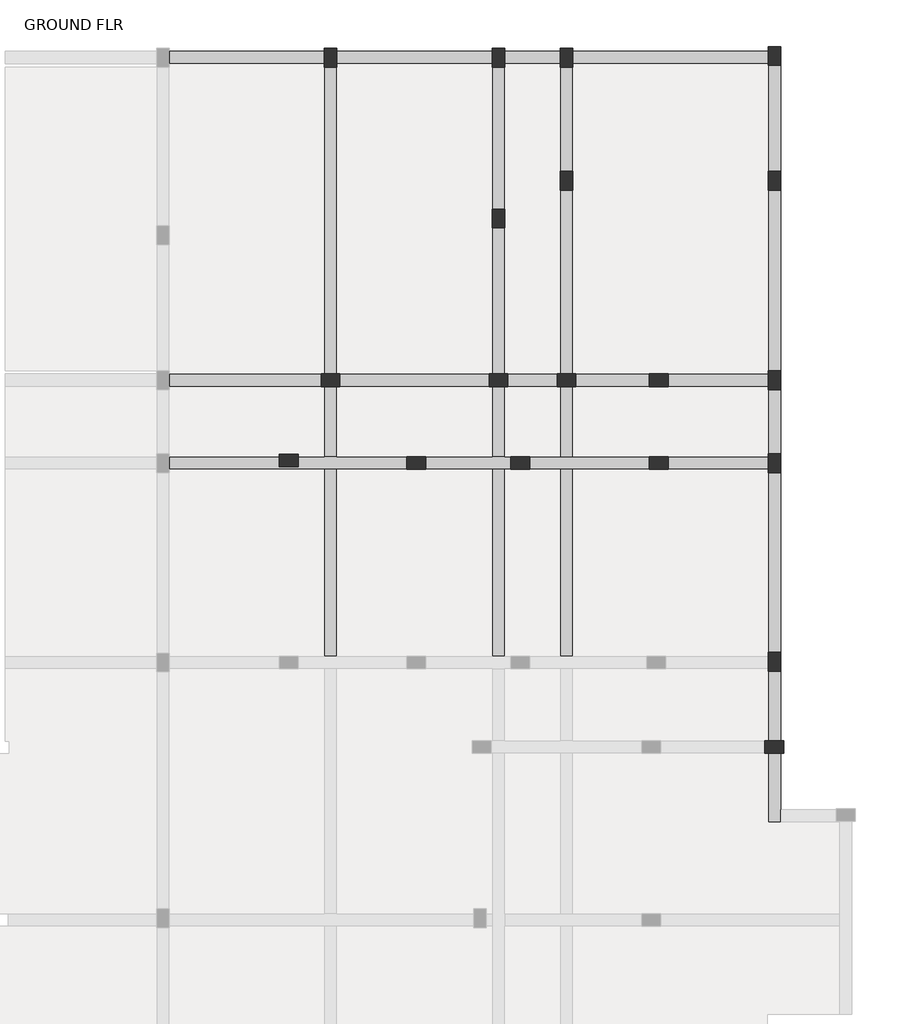
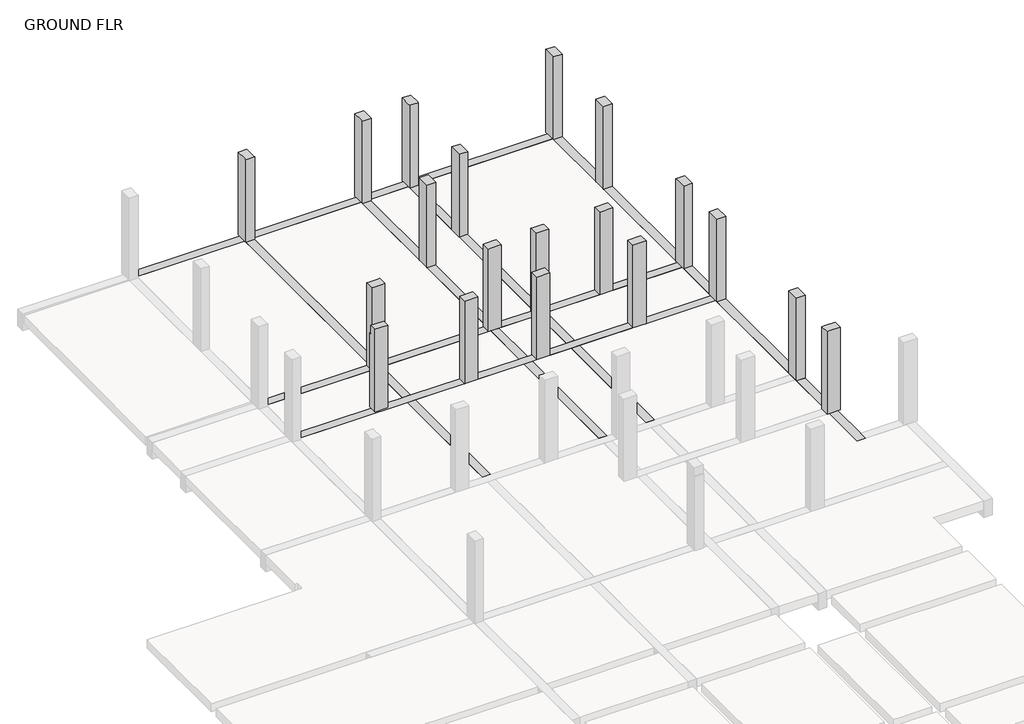
# One storey, part 5 of 5: 30 beams, 19 columns.
"""IFC4 building model written with IfcOpenShell, lengths in millimetres."""

from ifc_helpers import new_model, si_unit, frame, origin, origin_with_axes, place, context, project, spatial, polyline, outline, extrude, faceted_brep, element, save

model = new_model("IFC4")

# Units and contexts
model_context = context("Model", 3, world=origin())
ifc_project = project(units=[si_unit("LENGTHUNIT", "METRE", prefix="MILLI")], contexts=[model_context])

# Site, building, storey
site = spatial("IfcSite", under=ifc_project)
building = spatial("IfcBuilding", under=site)
storey = spatial("IfcBuildingStorey", under=building, Name="GROUND FLR", Elevation=0.0)

# Beams
placement = place(None, origin())
element("IfcBeam", 1, ObjectType="M_Concrete-Rectangular Beam : 300 x 600mm", at=placement, inside=storey, context=model_context, shape_type="Brep", body=[
    faceted_brep([(2024.7296816, 21537.8349362, 0.0), (2024.7296816, 21837.8349362, 0.0), (-1671.7865686, 21837.8349362, 0.0), (-1671.7865686, 21537.8349362, 0.0), (2024.7296816, 21537.8349362, -600.0), (2024.7296816, 21537.8349362, -300.0), (-1671.7865686, 21537.8349362, -300.0), (-1671.7865686, 21537.8349362, -600.0), (2024.7296816, 21837.8349362, -600.0), (-1671.7865686, 21837.8349362, -600.0)], [[[0, 1, 2, 3]], [[4, 5, 0, 3, 6, 7]], [[8, 4, 7, 9]], [[1, 8, 9, 2]], [[2, 9, 7, 6, 3]], [[1, 0, 5, 4, 8]]]),
])
element("IfcBeam", 2, ObjectType="M_Concrete-Rectangular Beam : 300 x 600mm", at=placement, inside=storey, context=model_context, shape_type="Brep", body=[
    faceted_brep([(6032.5248054, 21537.8349362, 0.0), (6032.5248054, 21837.8349362, 0.0), (2324.7296816, 21837.8349362, 0.0), (2324.7296816, 21537.8349362, 0.0), (6032.5248054, 21537.8349362, -600.0), (6032.5248054, 21537.8349362, -300.0), (2324.7296816, 21537.8349362, -300.0), (2324.7296816, 21537.8349362, -600.0), (6032.5248054, 21837.8349362, -600.0), (2324.7296816, 21837.8349362, -600.0)], [[[0, 1, 2, 3]], [[4, 5, 0, 3, 6, 7]], [[8, 4, 7, 9]], [[1, 8, 9, 2]], [[2, 9, 7, 6, 3]], [[1, 0, 5, 4, 8]]]),
])
element("IfcBeam", 3, ObjectType="M_Concrete-Rectangular Beam : 300 x 600mm", at=placement, inside=storey, context=model_context, shape_type="Brep", body=[
    faceted_brep([(7656.8679014, 21537.8349362, 0.0), (7656.8679014, 21837.8349362, 0.0), (6332.5248054, 21837.8349362, 0.0), (6332.5248054, 21537.8349362, 0.0), (7656.8679014, 21537.8349362, -600.0), (7656.8679014, 21537.8349362, -300.0), (6332.5248054, 21537.8349362, -300.0), (6332.5248054, 21537.8349362, -600.0), (7656.8679014, 21837.8349362, -600.0), (6332.5248054, 21837.8349362, -600.0)], [[[0, 1, 2, 3]], [[4, 5, 0, 3, 6, 7]], [[8, 4, 7, 9]], [[1, 8, 9, 2]], [[2, 9, 7, 6, 3]], [[1, 0, 5, 4, 8]]]),
])
element("IfcBeam", 4, ObjectType="M_Concrete-Rectangular Beam : 300 x 600mm", at=placement, inside=storey, context=model_context, shape_type="Brep", body=[
    faceted_brep([(7956.8679014, 21837.8349362, 0.0), (7956.8679014, 21537.8349362, 0.0), (12619.1163908, 21537.8349362, 0.0), (12619.1163908, 21837.8349362, 0.0), (7956.8679014, 21537.8349362, -300.0), (7956.8679014, 21537.8349362, -600.0), (12619.1163908, 21537.8349362, -600.0), (12619.1163908, 21537.8349362, -300.0), (7956.8679014, 21837.8349362, -600.0), (12619.1163908, 21837.8349362, -600.0)], [[[0, 1, 2, 3]], [[1, 4, 5, 6, 7, 2]], [[5, 8, 9, 6]], [[8, 0, 3, 9]], [[0, 8, 5, 4, 1]], [[3, 2, 7, 6, 9]]]),
])
element("IfcBeam", 5, ObjectType="M_Concrete-Rectangular Beam : 300 x 600mm", at=placement, inside=storey, context=model_context, shape_type="Brep", body=[
    faceted_brep([(12916.8679014, 5087.6057249, 0.0), (12616.8679014, 5087.6057249, 0.0), (12616.8679014, 3435.7536525, 0.0), (12916.8679014, 3435.7536525, 0.0), (12916.8679014, 3735.7536525, 0.0), (12616.8679014, 5087.6057249, -300.0), (12616.8679014, 5087.6057249, -600.0), (12616.8679014, 3435.7536525, -600.0), (12616.8679014, 3435.7536525, -300.0), (12916.8679014, 5087.6057249, -600.0), (12916.8679014, 3735.7536525, -600.0), (12916.8679014, 3435.7536525, -600.0), (12916.8679014, 3435.7536525, -300.0)], [[[0, 1, 2, 3, 4]], [[2, 1, 5, 6, 7, 8]], [[6, 9, 10, 11, 7]], [[9, 0, 4, 3, 12, 11, 10]], [[0, 9, 6, 5, 1]], [[3, 2, 8, 7, 11, 12]]]),
])
element("IfcBeam", 6, ObjectType="M_Concrete-Rectangular Beam : 300 x 600mm", at=placement, inside=storey, context=model_context, shape_type="Brep", body=[
    faceted_brep([(12616.8679014, 5387.6057249, 0.0), (12916.8679014, 5387.6057249, 0.0), (12916.8679014, 7044.7076276, 0.0), (12619.1163908, 7044.7076276, 0.0), (12619.1163908, 7399.7076276, 0.0), (12616.8679014, 7399.7076276, 0.0), (12616.8679014, 7099.7076276, 0.0), (12616.8679014, 7399.7076276, -600.0), (12616.8679014, 7099.7076276, -600.0), (12616.8679014, 5387.6057249, -600.0), (12616.8679014, 5387.6057249, -300.0), (12616.8679014, 7399.7076276, -300.0), (12916.8679014, 5387.6057249, -600.0), (12619.1163908, 7399.7076276, -600.0), (12619.1163908, 7044.7076276, -600.0), (12916.8679014, 7044.7076276, -600.0)], [[[0, 1, 2, 3, 4, 5, 6]], [[7, 8, 9, 10, 0, 6, 5, 11]], [[12, 9, 8, 7, 13, 14, 15]], [[1, 12, 15, 2]], [[1, 0, 10, 9, 12]], [[14, 3, 2, 15]], [[3, 14, 13, 4]], [[5, 4, 13, 7, 11]]]),
])
element("IfcBeam", 7, ObjectType="M_Concrete-Rectangular Beam : 300 x 600mm", at=placement, inside=storey, context=model_context, shape_type="SweptSolid", body=[
    extrude(outline(polyline([(12619.1163908, 11782.4075451), (12919.1163908, 11782.4075451), (12919.1163908, 7494.7076276), (12619.1163908, 7494.7076276), (12619.1163908, 11782.4075451)])), frame((0.0, 0.0, -600.0), z_axis=(0.0, 0.0, 1.0), x_axis=(1.0, 0.0, 0.0)), (0.0, 0.0, 1.0), 600.0),
])
element("IfcBeam", 8, ObjectType="M_Concrete-Rectangular Beam : 300 x 600mm", at=placement, inside=storey, context=model_context, shape_type="Brep", body=[
    faceted_brep([(12619.1163908, 13762.5179708, 0.0), (12619.1163908, 12232.4075451, 0.0), (12919.1163908, 12232.4075451, 0.0), (12919.1163908, 13762.5179708, 0.0), (12919.1163908, 12232.4075451, -600.0), (12919.1163908, 13762.5179708, -600.0), (12619.1163908, 12232.4075451, -600.0), (12619.1163908, 13762.5179708, -600.0), (12619.1163908, 13762.5179708, -300.0), (12619.1163908, 12232.4075451, -300.0)], [[[0, 1, 2, 3]], [[3, 2, 4, 5]], [[5, 4, 6, 7]], [[1, 0, 8, 7, 6, 9]], [[0, 3, 5, 7, 8]], [[6, 4, 2, 1, 9]]]),
])
element("IfcBeam", 9, ObjectType="M_Concrete-Rectangular Beam : 300 x 600mm", at=placement, inside=storey, context=model_context, shape_type="Brep", body=[
    faceted_brep([(12619.1163908, 18524.7148651, 0.0), (12619.1163908, 14212.5179708, 0.0), (12919.1163908, 14212.5179708, 0.0), (12919.1163908, 18524.7148651, 0.0), (12919.1163908, 14212.5179708, -600.0), (12919.1163908, 18524.7148651, -600.0), (12619.1163908, 14212.5179708, -600.0), (12619.1163908, 18524.7148651, -600.0), (12619.1163908, 18524.7148651, -300.0), (12619.1163908, 14212.5179708, -300.0)], [[[0, 1, 2, 3]], [[3, 2, 4, 5]], [[5, 4, 6, 7]], [[1, 0, 8, 7, 6, 9]], [[0, 3, 5, 7, 8]], [[6, 4, 2, 1, 9]]]),
])
element("IfcBeam", 10, ObjectType="M_Concrete-Rectangular Beam : 300 x 600mm", at=placement, inside=storey, context=model_context, shape_type="Brep", body=[
    faceted_brep([(12619.1163908, 21502.8349362, 0.0), (12619.1163908, 18974.7148651, 0.0), (12919.1163908, 18974.7148651, 0.0), (12919.1163908, 21502.8349362, 0.0), (12919.1163908, 18974.7148651, -600.0), (12919.1163908, 21502.8349362, -600.0), (12619.1163908, 18974.7148651, -600.0), (12619.1163908, 21502.8349362, -600.0), (12619.1163908, 21502.8349362, -300.0), (12619.1163908, 18974.7148651, -300.0)], [[[0, 1, 2, 3]], [[3, 2, 4, 5]], [[5, 4, 6, 7]], [[1, 0, 8, 7, 6, 9]], [[6, 4, 2, 1, 9]], [[0, 3, 5, 7, 8]]]),
])
element("IfcBeam", 11, ObjectType="M_Concrete-Rectangular Beam : 300 x 600mm", at=placement, inside=storey, context=model_context, shape_type="Brep", body=[
    faceted_brep([(2324.7296816, 21462.8349362, 0.0), (2024.7296816, 21462.8349362, 0.0), (2024.7296816, 14137.5179708, 0.0), (2324.7296816, 14137.5179708, 0.0), (2024.7296816, 21462.8349362, -300.0), (2024.7296816, 21462.8349362, -600.0), (2024.7296816, 14137.5179708, -600.0), (2024.7296816, 14137.5179708, -300.0), (2324.7296816, 21462.8349362, -600.0), (2324.7296816, 14137.5179708, -600.0), (2324.7296816, 14137.5179708, -300.0), (2324.7296816, 21462.8349362, -300.0)], [[[0, 1, 2, 3]], [[2, 1, 4, 5, 6, 7]], [[5, 8, 9, 6]], [[0, 3, 10, 9, 8, 11]], [[1, 0, 11, 8, 5, 4]], [[3, 2, 7, 6, 9, 10]]]),
])
element("IfcBeam", 12, ObjectType="M_Concrete-Rectangular Beam : 300 x 600mm", at=placement, inside=storey, context=model_context, shape_type="Brep", body=[
    faceted_brep([(2324.7296816, 13837.5179708, 0.0), (2024.7296816, 13837.5179708, 0.0), (2024.7296816, 12157.4075451, 0.0), (2324.7296816, 12157.4075451, 0.0), (2024.7296816, 13837.5179708, -300.0), (2024.7296816, 13837.5179708, -600.0), (2024.7296816, 12157.4075451, -600.0), (2024.7296816, 12157.4075451, -300.0), (2324.7296816, 13837.5179708, -600.0), (2324.7296816, 12157.4075451, -600.0), (2324.7296816, 12157.4075451, -300.0), (2324.7296816, 13837.5179708, -300.0)], [[[0, 1, 2, 3]], [[2, 1, 4, 5, 6, 7]], [[5, 8, 9, 6]], [[0, 3, 10, 9, 8, 11]], [[1, 0, 11, 8, 5, 4]], [[3, 2, 7, 6, 9, 10]]]),
])
element("IfcBeam", 13, ObjectType="M_Concrete-Rectangular Beam : 300 x 600mm", at=placement, inside=storey, context=model_context, shape_type="Brep", body=[
    faceted_brep([(6332.5248054, 21462.8349362, 0.0), (6032.5248054, 21462.8349362, 0.0), (6032.5248054, 18074.7148651, 0.0), (6332.5248054, 18074.7148651, 0.0), (6032.5248054, 21462.8349362, -300.0), (6032.5248054, 21462.8349362, -600.0), (6032.5248054, 18074.7148651, -600.0), (6032.5248054, 18074.7148651, -300.0), (6332.5248054, 21462.8349362, -600.0), (6332.5248054, 18074.7148651, -600.0), (6332.5248054, 18074.7148651, -300.0), (6332.5248054, 21462.8349362, -300.0)], [[[0, 1, 2, 3]], [[2, 1, 4, 5, 6, 7]], [[5, 8, 9, 6]], [[0, 3, 10, 9, 8, 11]], [[1, 0, 11, 8, 5, 4]], [[3, 2, 7, 6, 9, 10]]]),
])
element("IfcBeam", 14, ObjectType="M_Concrete-Rectangular Beam : 300 x 600mm", at=placement, inside=storey, context=model_context, shape_type="Brep", body=[
    faceted_brep([(6332.5248054, 17624.7148651, 0.0), (6032.5248054, 17624.7148651, 0.0), (6032.5248054, 14137.5179708, 0.0), (6332.5248054, 14137.5179708, 0.0), (6032.5248054, 17624.7148651, -300.0), (6032.5248054, 17624.7148651, -600.0), (6032.5248054, 14137.5179708, -600.0), (6032.5248054, 14137.5179708, -300.0), (6332.5248054, 17624.7148651, -600.0), (6332.5248054, 14137.5179708, -600.0), (6332.5248054, 14137.5179708, -300.0), (6332.5248054, 17624.7148651, -300.0)], [[[0, 1, 2, 3]], [[2, 1, 4, 5, 6, 7]], [[5, 8, 9, 6]], [[0, 3, 10, 9, 8, 11]], [[1, 0, 11, 8, 5, 4]], [[3, 2, 7, 6, 9, 10]]]),
])
element("IfcBeam", 15, ObjectType="M_Concrete-Rectangular Beam : 300 x 600mm", at=placement, inside=storey, context=model_context, shape_type="Brep", body=[
    faceted_brep([(6332.5248054, 13837.5179708, 0.0), (6032.5248054, 13837.5179708, 0.0), (6032.5248054, 12157.4075451, 0.0), (6332.5248054, 12157.4075451, 0.0), (6032.5248054, 13837.5179708, -300.0), (6032.5248054, 13837.5179708, -600.0), (6032.5248054, 12157.4075451, -600.0), (6032.5248054, 12157.4075451, -300.0), (6332.5248054, 13837.5179708, -600.0), (6332.5248054, 12157.4075451, -600.0), (6332.5248054, 12157.4075451, -300.0), (6332.5248054, 13837.5179708, -300.0)], [[[0, 1, 2, 3]], [[2, 1, 4, 5, 6, 7]], [[5, 8, 9, 6]], [[0, 3, 10, 9, 8, 11]], [[1, 0, 11, 8, 5, 4]], [[3, 2, 7, 6, 9, 10]]]),
])
element("IfcBeam", 16, ObjectType="M_Concrete-Rectangular Beam : 300 x 600mm", at=placement, inside=storey, context=model_context, shape_type="Brep", body=[
    faceted_brep([(7956.8679014, 21462.8349362, 0.0), (7656.8679014, 21462.8349362, 0.0), (7656.8679014, 18974.7148651, 0.0), (7956.8679014, 18974.7148651, 0.0), (7656.8679014, 21462.8349362, -300.0), (7656.8679014, 21462.8349362, -600.0), (7656.8679014, 18974.7148651, -600.0), (7656.8679014, 18974.7148651, -300.0), (7956.8679014, 21462.8349362, -600.0), (7956.8679014, 18974.7148651, -600.0), (7956.8679014, 18974.7148651, -300.0), (7956.8679014, 21462.8349362, -300.0)], [[[0, 1, 2, 3]], [[2, 1, 4, 5, 6, 7]], [[5, 8, 9, 6]], [[0, 3, 10, 9, 8, 11]], [[1, 0, 11, 8, 5, 4]], [[3, 2, 7, 6, 9, 10]]]),
])
element("IfcBeam", 17, ObjectType="M_Concrete-Rectangular Beam : 300 x 600mm", at=placement, inside=storey, context=model_context, shape_type="Brep", body=[
    faceted_brep([(7956.8679014, 18524.7148651, 0.0), (7656.8679014, 18524.7148651, 0.0), (7656.8679014, 14137.5179708, 0.0), (7956.8679014, 14137.5179708, 0.0), (7656.8679014, 18524.7148651, -300.0), (7656.8679014, 18524.7148651, -600.0), (7656.8679014, 14137.5179708, -600.0), (7656.8679014, 14137.5179708, -300.0), (7956.8679014, 18524.7148651, -600.0), (7956.8679014, 14137.5179708, -600.0), (7956.8679014, 14137.5179708, -300.0), (7956.8679014, 18524.7148651, -300.0)], [[[0, 1, 2, 3]], [[2, 1, 4, 5, 6, 7]], [[5, 8, 9, 6]], [[0, 3, 10, 9, 8, 11]], [[1, 0, 11, 8, 5, 4]], [[3, 2, 7, 6, 9, 10]]]),
])
element("IfcBeam", 18, ObjectType="M_Concrete-Rectangular Beam : 300 x 600mm", at=placement, inside=storey, context=model_context, shape_type="Brep", body=[
    faceted_brep([(7956.8679014, 13837.5179708, 0.0), (7656.8679014, 13837.5179708, 0.0), (7656.8679014, 12157.4075451, 0.0), (7956.8679014, 12157.4075451, 0.0), (7656.8679014, 13837.5179708, -300.0), (7656.8679014, 13837.5179708, -600.0), (7656.8679014, 12157.4075451, -600.0), (7656.8679014, 12157.4075451, -300.0), (7956.8679014, 13837.5179708, -600.0), (7956.8679014, 12157.4075451, -600.0), (7956.8679014, 12157.4075451, -300.0), (7956.8679014, 13837.5179708, -300.0)], [[[0, 1, 2, 3]], [[2, 1, 4, 5, 6, 7]], [[5, 8, 9, 6]], [[0, 3, 10, 9, 8, 11]], [[1, 0, 11, 8, 5, 4]], [[3, 2, 7, 6, 9, 10]]]),
])
element("IfcBeam", 19, ObjectType="M_Concrete-Rectangular Beam : 300 x 600mm", at=placement, inside=storey, context=model_context, shape_type="Brep", body=[
    faceted_brep([(-1671.7865686, 14137.5179708, 0.0), (-1671.7865686, 13837.5179708, 0.0), (1949.7296816, 13837.5179708, 0.0), (1949.7296816, 14137.5179708, 0.0), (-1671.7865686, 13837.5179708, -300.0), (-1671.7865686, 13837.5179708, -600.0), (1949.7296816, 13837.5179708, -600.0), (1949.7296816, 13837.5179708, -300.0), (-1671.7865686, 14137.5179708, -600.0), (1949.7296816, 14137.5179708, -600.0), (1949.7296816, 14137.5179708, -300.0), (-1671.7865686, 14137.5179708, -300.0)], [[[0, 1, 2, 3]], [[2, 1, 4, 5, 6, 7]], [[5, 8, 9, 6]], [[0, 3, 10, 9, 8, 11]], [[1, 0, 11, 8, 5, 4]], [[3, 2, 7, 6, 9, 10]]]),
])
element("IfcBeam", 20, ObjectType="M_Concrete-Rectangular Beam : 300 x 600mm", at=placement, inside=storey, context=model_context, shape_type="Brep", body=[
    faceted_brep([(2399.7296816, 14137.5179708, 0.0), (2399.7296816, 13837.5179708, 0.0), (5957.5248054, 13837.5179708, 0.0), (5957.5248054, 14137.5179708, 0.0), (2399.7296816, 13837.5179708, -300.0), (2399.7296816, 13837.5179708, -600.0), (5957.5248054, 13837.5179708, -600.0), (5957.5248054, 13837.5179708, -300.0), (2399.7296816, 14137.5179708, -600.0), (5957.5248054, 14137.5179708, -600.0), (5957.5248054, 14137.5179708, -300.0), (2399.7296816, 14137.5179708, -300.0)], [[[0, 1, 2, 3]], [[2, 1, 4, 5, 6, 7]], [[5, 8, 9, 6]], [[0, 3, 10, 9, 8, 11]], [[1, 0, 11, 8, 5, 4]], [[3, 2, 7, 6, 9, 10]]]),
])
element("IfcBeam", 21, ObjectType="M_Concrete-Rectangular Beam : 300 x 600mm", at=placement, inside=storey, context=model_context, shape_type="Brep", body=[
    faceted_brep([(6407.5248054, 14137.5179708, 0.0), (6407.5248054, 13837.5179708, 0.0), (7581.8679014, 13837.5179708, 0.0), (7581.8679014, 14137.5179708, 0.0), (6407.5248054, 13837.5179708, -300.0), (6407.5248054, 13837.5179708, -600.0), (7581.8679014, 13837.5179708, -600.0), (7581.8679014, 13837.5179708, -300.0), (6407.5248054, 14137.5179708, -600.0), (7581.8679014, 14137.5179708, -600.0), (7581.8679014, 14137.5179708, -300.0), (6407.5248054, 14137.5179708, -300.0)], [[[0, 1, 2, 3]], [[2, 1, 4, 5, 6, 7]], [[5, 8, 9, 6]], [[0, 3, 10, 9, 8, 11]], [[1, 0, 11, 8, 5, 4]], [[3, 2, 7, 6, 9, 10]]]),
])
element("IfcBeam", 22, ObjectType="M_Concrete-Rectangular Beam : 300 x 600mm", at=placement, inside=storey, context=model_context, shape_type="Brep", body=[
    faceted_brep([(8031.8679014, 14137.5179708, 0.0), (8031.8679014, 13837.5179708, 0.0), (9781.8679014, 13837.5179708, 0.0), (9781.8679014, 14137.5179708, 0.0), (8031.8679014, 13837.5179708, -300.0), (8031.8679014, 13837.5179708, -600.0), (9781.8679014, 13837.5179708, -600.0), (9781.8679014, 13837.5179708, -300.0), (8031.8679014, 14137.5179708, -600.0), (9781.8679014, 14137.5179708, -600.0), (9781.8679014, 14137.5179708, -300.0), (8031.8679014, 14137.5179708, -300.0)], [[[0, 1, 2, 3]], [[2, 1, 4, 5, 6, 7]], [[5, 8, 9, 6]], [[0, 3, 10, 9, 8, 11]], [[1, 0, 11, 8, 5, 4]], [[3, 2, 7, 6, 9, 10]]]),
])
element("IfcBeam", 23, ObjectType="M_Concrete-Rectangular Beam : 300 x 600mm", at=placement, inside=storey, context=model_context, shape_type="Brep", body=[
    faceted_brep([(10231.8679014, 14137.5179708, 0.0), (10231.8679014, 13837.5179708, 0.0), (12619.1163908, 13837.5179708, 0.0), (12619.1163908, 14137.5179708, 0.0), (10231.8679014, 13837.5179708, -300.0), (10231.8679014, 13837.5179708, -600.0), (12619.1163908, 13837.5179708, -600.0), (12619.1163908, 13837.5179708, -300.0), (10231.8679014, 14137.5179708, -600.0), (12619.1163908, 14137.5179708, -600.0), (12619.1163908, 14137.5179708, -300.0), (10231.8679014, 14137.5179708, -300.0)], [[[0, 1, 2, 3]], [[2, 1, 4, 5, 6, 7]], [[5, 8, 9, 6]], [[0, 3, 10, 9, 8, 11]], [[1, 0, 11, 8, 5, 4]], [[3, 2, 7, 6, 9, 10]]]),
])
element("IfcBeam", 24, ObjectType="M_Concrete-Rectangular Beam : 300 x 600mm", at=placement, inside=storey, context=model_context, shape_type="Brep", body=[
    faceted_brep([(-1671.7865686, 12157.4075451, 0.0), (-1671.7865686, 11857.4075451, 0.0), (2024.7296816, 11857.4075451, 0.0), (2324.7296816, 11857.4075451, 0.0), (3997.5248054, 11857.4075451, 0.0), (3997.5248054, 12157.4075451, 0.0), (2324.7296816, 12157.4075451, 0.0), (2024.7296816, 12157.4075451, 0.0), (1399.7296816, 12157.4075451, 0.0), (1399.7296816, 11917.4075451, 0.0), (949.7296816, 11917.4075451, 0.0), (949.7296816, 12157.4075451, 0.0), (-1671.7865686, 11857.4075451, -600.0), (2024.7296816, 11857.4075451, -600.0), (2324.7296816, 11857.4075451, -600.0), (3997.5248054, 11857.4075451, -600.0), (3997.5248054, 11857.4075451, -300.0), (-1671.7865686, 11857.4075451, -300.0), (-1671.7865686, 12157.4075451, -600.0), (949.7296816, 12157.4075451, -600.0), (949.7296816, 11917.4075451, -600.0), (1399.7296816, 11917.4075451, -600.0), (1399.7296816, 12157.4075451, -600.0), (2024.7296816, 12157.4075451, -600.0), (2324.7296816, 12157.4075451, -600.0), (3997.5248054, 12157.4075451, -600.0), (949.7296816, 12157.4075451, -300.0), (-1671.7865686, 12157.4075451, -300.0), (3997.5248054, 12157.4075451, -300.0), (1399.7296816, 12157.4075451, -300.0)], [[[0, 1, 2, 3, 4, 5, 6, 7, 8, 9, 10, 11]], [[12, 13, 14, 15, 16, 4, 3, 2, 1, 17]], [[12, 18, 19, 20, 21, 22, 23, 24, 25, 15, 14, 13]], [[0, 11, 26, 19, 18, 27]], [[1, 0, 27, 18, 12, 17]], [[5, 4, 16, 15, 25, 28]], [[20, 10, 9, 21]], [[10, 20, 19, 26, 11]], [[21, 9, 8, 29, 22]], [[25, 24, 23, 22, 29, 8, 7, 6, 5, 28]]]),
])
element("IfcBeam", 25, ObjectType="M_Concrete-Rectangular Beam : 300 x 600mm", at=placement, inside=storey, context=model_context, shape_type="Brep", body=[
    faceted_brep([(4447.5248054, 12157.4075451, 0.0), (4447.5248054, 11857.4075451, 0.0), (6032.5248054, 11857.4075451, 0.0), (6332.5248054, 11857.4075451, 0.0), (6481.8679014, 11857.4075451, 0.0), (6481.8679014, 12157.4075451, 0.0), (6332.5248054, 12157.4075451, 0.0), (6032.5248054, 12157.4075451, 0.0), (4447.5248054, 11857.4075451, -600.0), (6032.5248054, 11857.4075451, -600.0), (6332.5248054, 11857.4075451, -600.0), (6481.8679014, 11857.4075451, -600.0), (6481.8679014, 11857.4075451, -300.0), (4447.5248054, 11857.4075451, -300.0), (4447.5248054, 12157.4075451, -600.0), (6032.5248054, 12157.4075451, -600.0), (6332.5248054, 12157.4075451, -600.0), (6481.8679014, 12157.4075451, -600.0), (4447.5248054, 12157.4075451, -300.0), (6481.8679014, 12157.4075451, -300.0)], [[[0, 1, 2, 3, 4, 5, 6, 7]], [[8, 9, 10, 11, 12, 4, 3, 2, 1, 13]], [[8, 14, 15, 16, 17, 11, 10, 9]], [[17, 16, 15, 14, 18, 0, 7, 6, 5, 19]], [[1, 0, 18, 14, 8, 13]], [[5, 4, 12, 11, 17, 19]]]),
])
element("IfcBeam", 26, ObjectType="M_Concrete-Rectangular Beam : 300 x 600mm", at=placement, inside=storey, context=model_context, shape_type="Brep", body=[
    faceted_brep([(6931.8679014, 12157.4075451, 0.0), (6931.8679014, 11857.4075451, 0.0), (7656.8679014, 11857.4075451, 0.0), (7956.8679014, 11857.4075451, 0.0), (9781.8679014, 11857.4075451, 0.0), (9781.8679014, 12157.4075451, 0.0), (7956.8679014, 12157.4075451, 0.0), (7656.8679014, 12157.4075451, 0.0), (6931.8679014, 11857.4075451, -600.0), (7656.8679014, 11857.4075451, -600.0), (7956.8679014, 11857.4075451, -600.0), (9781.8679014, 11857.4075451, -600.0), (9781.8679014, 11857.4075451, -300.0), (6931.8679014, 11857.4075451, -300.0), (6931.8679014, 12157.4075451, -600.0), (7656.8679014, 12157.4075451, -600.0), (7956.8679014, 12157.4075451, -600.0), (9781.8679014, 12157.4075451, -600.0), (6931.8679014, 12157.4075451, -300.0), (9781.8679014, 12157.4075451, -300.0)], [[[0, 1, 2, 3, 4, 5, 6, 7]], [[8, 9, 10, 11, 12, 4, 3, 2, 1, 13]], [[8, 14, 15, 16, 17, 11, 10, 9]], [[17, 16, 15, 14, 18, 0, 7, 6, 5, 19]], [[1, 0, 18, 14, 8, 13]], [[5, 4, 12, 11, 17, 19]]]),
])
element("IfcBeam", 27, ObjectType="M_Concrete-Rectangular Beam : 300 x 600mm", at=placement, inside=storey, context=model_context, shape_type="Brep", body=[
    faceted_brep([(10231.8679014, 12157.4075451, 0.0), (10231.8679014, 11857.4075451, 0.0), (12616.8679014, 11857.4075451, 0.0), (12619.1163908, 11857.4075451, 0.0), (12619.1163908, 12157.4075451, 0.0), (10231.8679014, 11857.4075451, -600.0), (12619.1163908, 11857.4075451, -600.0), (10231.8679014, 11857.4075451, -300.0), (10231.8679014, 12157.4075451, -600.0), (12619.1163908, 12157.4075451, -600.0), (12619.1163908, 12157.4075451, -300.0), (10231.8679014, 12157.4075451, -300.0)], [[[0, 1, 2, 3, 4]], [[5, 6, 3, 2, 1, 7]], [[5, 8, 9, 6]], [[0, 4, 10, 9, 8, 11]], [[1, 0, 11, 8, 5, 7]], [[4, 3, 6, 9, 10]]]),
])
element("IfcBeam", 28, ObjectType="M_Concrete-Rectangular Beam : 300 x 600mm", at=placement, inside=storey, context=model_context, shape_type="Brep", body=[
    faceted_brep([(2324.7296816, 11857.4075451, 0.0), (2024.7296816, 11857.4075451, 0.0), (2024.7296816, 7399.7076276, 0.0), (2324.7296816, 7399.7076276, 0.0), (2024.7296816, 11857.4075451, -300.0), (2024.7296816, 11857.4075451, -600.0), (2024.7296816, 7399.7076276, -600.0), (2024.7296816, 7399.7076276, -300.0), (2324.7296816, 11857.4075451, -600.0), (2324.7296816, 7399.7076276, -600.0), (2324.7296816, 7399.7076276, -300.0), (2324.7296816, 11857.4075451, -300.0)], [[[0, 1, 2, 3]], [[2, 1, 4, 5, 6, 7]], [[5, 8, 9, 6]], [[0, 3, 10, 9, 8, 11]], [[1, 0, 11, 8, 5, 4]], [[3, 2, 7, 6, 9, 10]]]),
])
element("IfcBeam", 29, ObjectType="M_Concrete-Rectangular Beam : 300 x 600mm", at=placement, inside=storey, context=model_context, shape_type="Brep", body=[
    faceted_brep([(6332.5248054, 11857.4075451, 0.0), (6032.5248054, 11857.4075451, 0.0), (6032.5248054, 7399.7076276, 0.0), (6332.5248054, 7399.7076276, 0.0), (6032.5248054, 11857.4075451, -300.0), (6032.5248054, 11857.4075451, -600.0), (6032.5248054, 7399.7076276, -600.0), (6032.5248054, 7399.7076276, -300.0), (6332.5248054, 11857.4075451, -600.0), (6332.5248054, 7399.7076276, -600.0), (6332.5248054, 7399.7076276, -300.0), (6332.5248054, 11857.4075451, -300.0)], [[[0, 1, 2, 3]], [[2, 1, 4, 5, 6, 7]], [[5, 8, 9, 6]], [[0, 3, 10, 9, 8, 11]], [[1, 0, 11, 8, 5, 4]], [[3, 2, 7, 6, 9, 10]]]),
])
element("IfcBeam", 30, ObjectType="M_Concrete-Rectangular Beam : 300 x 600mm", at=placement, inside=storey, context=model_context, shape_type="Brep", body=[
    faceted_brep([(7956.8679014, 11857.4075451, 0.0), (7656.8679014, 11857.4075451, 0.0), (7656.8679014, 7399.7076276, 0.0), (7956.8679014, 7399.7076276, 0.0), (7656.8679014, 11857.4075451, -300.0), (7656.8679014, 11857.4075451, -600.0), (7656.8679014, 7399.7076276, -600.0), (7656.8679014, 7399.7076276, -300.0), (7956.8679014, 11857.4075451, -600.0), (7956.8679014, 7399.7076276, -600.0), (7956.8679014, 7399.7076276, -300.0), (7956.8679014, 11857.4075451, -300.0)], [[[0, 1, 2, 3]], [[2, 1, 4, 5, 6, 7]], [[5, 8, 9, 6]], [[0, 3, 10, 9, 8, 11]], [[1, 0, 11, 8, 5, 4]], [[3, 2, 7, 6, 9, 10]]]),
])

# Columns
element("IfcColumn", 31, ObjectType="M_Concrete-Rectangular-Column : 300 x 450mm", at=placement, inside=storey, context=model_context, shape_type="Brep", body=[
    faceted_brep([(2324.7296816, 21912.8349362, 0.0), (2324.7296816, 21462.8349362, 0.0), (2024.7296816, 21462.8349362, 0.0), (2024.7296816, 21912.8349362, 0.0), (2324.7296816, 21912.8349362, 3000.0), (2324.7296816, 21537.8349362, 3000.0), (2324.7296816, 21462.8349362, 3000.0), (2324.7296816, 21462.8349362, 2700.0), (2024.7296816, 21462.8349362, 3000.0), (2024.7296816, 21462.8349362, 2700.0), (2024.7296816, 21537.8349362, 3000.0), (2024.7296816, 21912.8349362, 3000.0)], [[[0, 1, 2, 3]], [[1, 0, 4, 5, 6, 7]], [[2, 1, 7, 6, 8, 9]], [[3, 2, 9, 8, 10, 11]], [[0, 3, 11, 4]], [[8, 6, 5, 4, 11, 10]]]),
])
element("IfcColumn", 32, ObjectType="M_Concrete-Rectangular-Column : 300 x 450mm", at=placement, inside=storey, context=model_context, shape_type="Brep", body=[
    faceted_brep([(6332.5248054, 21912.8349362, 0.0), (6332.5248054, 21462.8349362, 0.0), (6032.5248054, 21462.8349362, 0.0), (6032.5248054, 21912.8349362, 0.0), (6332.5248054, 21912.8349362, 3000.0), (6332.5248054, 21537.8349362, 3000.0), (6332.5248054, 21462.8349362, 3000.0), (6332.5248054, 21462.8349362, 2700.0), (6032.5248054, 21462.8349362, 3000.0), (6032.5248054, 21462.8349362, 2700.0), (6032.5248054, 21537.8349362, 3000.0), (6032.5248054, 21912.8349362, 3000.0)], [[[0, 1, 2, 3]], [[1, 0, 4, 5, 6, 7]], [[2, 1, 7, 6, 8, 9]], [[3, 2, 9, 8, 10, 11]], [[0, 3, 11, 4]], [[8, 6, 5, 4, 11, 10]]]),
])
element("IfcColumn", 33, ObjectType="M_Concrete-Rectangular-Column : 300 x 450mm", at=placement, inside=storey, context=model_context, shape_type="Brep", body=[
    faceted_brep([(7956.8679014, 21912.8349362, 0.0), (7956.8679014, 21462.8349362, 0.0), (7656.8679014, 21462.8349362, 0.0), (7656.8679014, 21912.8349362, 0.0), (7956.8679014, 21912.8349362, 3000.0), (7956.8679014, 21537.8349362, 3000.0), (7956.8679014, 21462.8349362, 3000.0), (7956.8679014, 21462.8349362, 2700.0), (7656.8679014, 21462.8349362, 3000.0), (7656.8679014, 21462.8349362, 2700.0), (7656.8679014, 21537.8349362, 3000.0), (7656.8679014, 21912.8349362, 3000.0)], [[[0, 1, 2, 3]], [[1, 0, 4, 5, 6, 7]], [[2, 1, 7, 6, 8, 9]], [[3, 2, 9, 8, 10, 11]], [[0, 3, 11, 4]], [[8, 6, 5, 4, 11, 10]]]),
])
element("IfcColumn", 34, ObjectType="M_Concrete-Rectangular-Column : 300 x 450mm", at=placement, inside=storey, context=model_context, shape_type="Brep", body=[
    faceted_brep([(12919.1163908, 21952.8349362, 0.0), (12919.1163908, 21502.8349362, 0.0), (12619.1163908, 21502.8349362, 0.0), (12619.1163908, 21952.8349362, 0.0), (12919.1163908, 21952.8349362, 3000.0), (12919.1163908, 21502.8349362, 3000.0), (12619.1163908, 21502.8349362, 3000.0), (12619.1163908, 21502.8349362, 2700.0), (12619.1163908, 21537.8349362, 3000.0), (12619.1163908, 21952.8349362, 3000.0)], [[[0, 1, 2, 3]], [[1, 0, 4, 5]], [[2, 1, 5, 6, 7]], [[3, 2, 7, 6, 8, 9]], [[0, 3, 9, 4]], [[5, 4, 9, 8, 6]]]),
])
element("IfcColumn", 35, ObjectType="M_Concrete-Rectangular-Column : 300 x 450mm", at=placement, inside=storey, context=model_context, shape_type="Brep", body=[
    faceted_brep([(12919.1163908, 18974.7148651, 0.0), (12919.1163908, 18524.7148651, 0.0), (12619.1163908, 18524.7148651, 0.0), (12619.1163908, 18974.7148651, 0.0), (12919.1163908, 18974.7148651, 3000.0), (12919.1163908, 18524.7148651, 3000.0), (12619.1163908, 18524.7148651, 3000.0), (12619.1163908, 18524.7148651, 2700.0), (12619.1163908, 18974.7148651, 3000.0), (12619.1163908, 18974.7148651, 2700.0)], [[[0, 1, 2, 3]], [[1, 0, 4, 5]], [[2, 1, 5, 6, 7]], [[3, 2, 7, 6, 8, 9]], [[0, 3, 9, 8, 4]], [[5, 4, 8, 6]]]),
])
element("IfcColumn", 36, ObjectType="M_Concrete-Rectangular-Column : 300 x 450mm", at=placement, inside=storey, context=model_context, shape_type="Brep", body=[
    faceted_brep([(7956.8679014, 18974.7148651, 0.0), (7956.8679014, 18524.7148651, 0.0), (7656.8679014, 18524.7148651, 0.0), (7656.8679014, 18974.7148651, 0.0), (7956.8679014, 18974.7148651, 2700.0), (7956.8679014, 18974.7148651, 3000.0), (7956.8679014, 18524.7148651, 3000.0), (7956.8679014, 18524.7148651, 2700.0), (7656.8679014, 18524.7148651, 3000.0), (7656.8679014, 18524.7148651, 2700.0), (7656.8679014, 18974.7148651, 3000.0), (7656.8679014, 18974.7148651, 2700.0)], [[[0, 1, 2, 3]], [[1, 0, 4, 5, 6, 7]], [[2, 1, 7, 6, 8, 9]], [[3, 2, 9, 8, 10, 11]], [[0, 3, 11, 10, 5, 4]], [[6, 5, 10, 8]]]),
])
element("IfcColumn", 37, ObjectType="M_Concrete-Rectangular-Column : 300 x 450mm", at=placement, inside=storey, context=model_context, shape_type="Brep", body=[
    faceted_brep([(6332.5248054, 18074.7148651, 0.0), (6332.5248054, 17624.7148651, 0.0), (6032.5248054, 17624.7148651, 0.0), (6032.5248054, 18074.7148651, 0.0), (6332.5248054, 18074.7148651, 2700.0), (6332.5248054, 18074.7148651, 3000.0), (6332.5248054, 17624.7148651, 3000.0), (6332.5248054, 17624.7148651, 2700.0), (6032.5248054, 17624.7148651, 3000.0), (6032.5248054, 17624.7148651, 2700.0), (6032.5248054, 18074.7148651, 3000.0), (6032.5248054, 18074.7148651, 2700.0)], [[[0, 1, 2, 3]], [[1, 0, 4, 5, 6, 7]], [[2, 1, 7, 6, 8, 9]], [[3, 2, 9, 8, 10, 11]], [[0, 3, 11, 10, 5, 4]], [[6, 5, 10, 8]]]),
])
element("IfcColumn", 38, ObjectType="M_Concrete-Rectangular-Column : 300 x 450mm", at=placement, inside=storey, context=model_context, shape_type="Brep", body=[
    faceted_brep([(1949.7296816, 14137.5179708, 0.0), (2399.7296816, 14137.5179708, 0.0), (2399.7296816, 13837.5179708, 0.0), (1949.7296816, 13837.5179708, 0.0), (1949.7296816, 14137.5179708, 2700.0), (1949.7296816, 14137.5179708, 3000.0), (2024.7296816, 14137.5179708, 3000.0), (2324.7296816, 14137.5179708, 3000.0), (2399.7296816, 14137.5179708, 3000.0), (2399.7296816, 14137.5179708, 2700.0), (2399.7296816, 13837.5179708, 3000.0), (2399.7296816, 13837.5179708, 2700.0), (2324.7296816, 13837.5179708, 3000.0), (2024.7296816, 13837.5179708, 3000.0), (1949.7296816, 13837.5179708, 3000.0), (1949.7296816, 13837.5179708, 2700.0)], [[[0, 1, 2, 3]], [[1, 0, 4, 5, 6, 7, 8, 9]], [[2, 1, 9, 8, 10, 11]], [[3, 2, 11, 10, 12, 13, 14, 15]], [[0, 3, 15, 14, 5, 4]], [[10, 8, 7, 6, 5, 14, 13, 12]]]),
])
element("IfcColumn", 39, ObjectType="M_Concrete-Rectangular-Column : 300 x 450mm", at=placement, inside=storey, context=model_context, shape_type="Brep", body=[
    faceted_brep([(5957.5248054, 14137.5179708, 0.0), (6407.5248054, 14137.5179708, 0.0), (6407.5248054, 13837.5179708, 0.0), (5957.5248054, 13837.5179708, 0.0), (5957.5248054, 14137.5179708, 2700.0), (5957.5248054, 14137.5179708, 3000.0), (6032.5248054, 14137.5179708, 3000.0), (6332.5248054, 14137.5179708, 3000.0), (6407.5248054, 14137.5179708, 3000.0), (6407.5248054, 14137.5179708, 2700.0), (6407.5248054, 13837.5179708, 3000.0), (6407.5248054, 13837.5179708, 2700.0), (6332.5248054, 13837.5179708, 3000.0), (6032.5248054, 13837.5179708, 3000.0), (5957.5248054, 13837.5179708, 3000.0), (5957.5248054, 13837.5179708, 2700.0)], [[[0, 1, 2, 3]], [[1, 0, 4, 5, 6, 7, 8, 9]], [[2, 1, 9, 8, 10, 11]], [[3, 2, 11, 10, 12, 13, 14, 15]], [[0, 3, 15, 14, 5, 4]], [[10, 8, 7, 6, 5, 14, 13, 12]]]),
])
element("IfcColumn", 40, ObjectType="M_Concrete-Rectangular-Column : 300 x 450mm", at=placement, inside=storey, context=model_context, shape_type="Brep", body=[
    faceted_brep([(7581.8679014, 14137.5179708, 0.0), (8031.8679014, 14137.5179708, 0.0), (8031.8679014, 13837.5179708, 0.0), (7581.8679014, 13837.5179708, 0.0), (7581.8679014, 14137.5179708, 2700.0), (7581.8679014, 14137.5179708, 3000.0), (7656.8679014, 14137.5179708, 3000.0), (7956.8679014, 14137.5179708, 3000.0), (8031.8679014, 14137.5179708, 3000.0), (8031.8679014, 14137.5179708, 2700.0), (8031.8679014, 13837.5179708, 3000.0), (8031.8679014, 13837.5179708, 2700.0), (7956.8679014, 13837.5179708, 3000.0), (7656.8679014, 13837.5179708, 3000.0), (7581.8679014, 13837.5179708, 3000.0), (7581.8679014, 13837.5179708, 2700.0)], [[[0, 1, 2, 3]], [[1, 0, 4, 5, 6, 7, 8, 9]], [[2, 1, 9, 8, 10, 11]], [[3, 2, 11, 10, 12, 13, 14, 15]], [[0, 3, 15, 14, 5, 4]], [[10, 8, 7, 6, 5, 14, 13, 12]]]),
])
element("IfcColumn", 41, ObjectType="M_Concrete-Rectangular-Column : 300 x 450mm", at=placement, inside=storey, context=model_context, shape_type="Brep", body=[
    faceted_brep([(9781.8679014, 14137.5179708, 0.0), (10231.8679014, 14137.5179708, 0.0), (10231.8679014, 13837.5179708, 0.0), (9781.8679014, 13837.5179708, 0.0), (9781.8679014, 14137.5179708, 2700.0), (9781.8679014, 14137.5179708, 3000.0), (10231.8679014, 14137.5179708, 3000.0), (10231.8679014, 14137.5179708, 2700.0), (10231.8679014, 13837.5179708, 3000.0), (10231.8679014, 13837.5179708, 2700.0), (9781.8679014, 13837.5179708, 3000.0), (9781.8679014, 13837.5179708, 2700.0)], [[[0, 1, 2, 3]], [[1, 0, 4, 5, 6, 7]], [[2, 1, 7, 6, 8, 9]], [[3, 2, 9, 8, 10, 11]], [[0, 3, 11, 10, 5, 4]], [[6, 5, 10, 8]]]),
])
element("IfcColumn", 42, ObjectType="M_Concrete-Rectangular-Column : 300 x 450mm", at=placement, inside=storey, context=model_context, shape_type="Brep", body=[
    faceted_brep([(12619.1163908, 13762.5179708, 0.0), (12619.1163908, 14212.5179708, 0.0), (12919.1163908, 14212.5179708, 0.0), (12919.1163908, 13762.5179708, 0.0), (12619.1163908, 13762.5179708, 2700.0), (12619.1163908, 13762.5179708, 3000.0), (12619.1163908, 13837.5179708, 3000.0), (12619.1163908, 14137.5179708, 3000.0), (12619.1163908, 14212.5179708, 3000.0), (12619.1163908, 14212.5179708, 2700.0), (12919.1163908, 14212.5179708, 3000.0), (12919.1163908, 13762.5179708, 3000.0)], [[[0, 1, 2, 3]], [[1, 0, 4, 5, 6, 7, 8, 9]], [[2, 1, 9, 8, 10]], [[3, 2, 10, 11]], [[0, 3, 11, 5, 4]], [[10, 8, 7, 6, 5, 11]]]),
])
element("IfcColumn", 43, ObjectType="M_Concrete-Rectangular-Column : 300 x 450mm", at=placement, inside=storey, context=model_context, shape_type="Brep", body=[
    faceted_brep([(1399.7296816, 11917.4075451, 0.0), (949.7296816, 11917.4075451, 0.0), (949.7296816, 12217.4075451, 0.0), (1399.7296816, 12217.4075451, 0.0), (1399.7296816, 11917.4075451, 2400.0), (1399.7296816, 11917.4075451, 3000.0), (949.7296816, 11917.4075451, 3000.0), (949.7296816, 11917.4075451, 2400.0), (949.7296816, 12157.4075451, 3000.0), (949.7296816, 12157.4075451, 2700.0), (949.7296816, 12217.4075451, 2700.0), (1399.7296816, 12217.4075451, 2700.0), (1399.7296816, 12157.4075451, 2700.0), (1399.7296816, 12157.4075451, 3000.0)], [[[0, 1, 2, 3]], [[1, 0, 4, 5, 6, 7]], [[2, 1, 7, 6, 8, 9, 10]], [[3, 2, 10, 11]], [[0, 3, 11, 12, 13, 5, 4]], [[6, 5, 13, 8]], [[9, 12, 11, 10]], [[12, 9, 8, 13]]]),
])
element("IfcColumn", 44, ObjectType="M_Concrete-Rectangular-Column : 300 x 450mm", at=placement, inside=storey, context=model_context, shape_type="Brep", body=[
    faceted_brep([(4447.5248054, 11857.4075451, 0.0), (3997.5248054, 11857.4075451, 0.0), (3997.5248054, 12157.4075451, 0.0), (4447.5248054, 12157.4075451, 0.0), (4447.5248054, 11857.4075451, 2700.0), (4447.5248054, 11857.4075451, 3000.0), (3997.5248054, 11857.4075451, 3000.0), (3997.5248054, 11857.4075451, 2700.0), (3997.5248054, 12157.4075451, 3000.0), (3997.5248054, 12157.4075451, 2700.0), (4447.5248054, 12157.4075451, 3000.0), (4447.5248054, 12157.4075451, 2700.0)], [[[0, 1, 2, 3]], [[1, 0, 4, 5, 6, 7]], [[2, 1, 7, 6, 8, 9]], [[3, 2, 9, 8, 10, 11]], [[0, 3, 11, 10, 5, 4]], [[6, 5, 10, 8]]]),
])
element("IfcColumn", 45, ObjectType="M_Concrete-Rectangular-Column : 300 x 450mm", at=placement, inside=storey, context=model_context, shape_type="Brep", body=[
    faceted_brep([(6931.8679014, 11857.4075451, 0.0), (6481.8679014, 11857.4075451, 0.0), (6481.8679014, 12157.4075451, 0.0), (6931.8679014, 12157.4075451, 0.0), (6931.8679014, 11857.4075451, 2700.0), (6931.8679014, 11857.4075451, 3000.0), (6481.8679014, 11857.4075451, 3000.0), (6481.8679014, 11857.4075451, 2700.0), (6481.8679014, 12157.4075451, 3000.0), (6481.8679014, 12157.4075451, 2700.0), (6931.8679014, 12157.4075451, 3000.0), (6931.8679014, 12157.4075451, 2700.0)], [[[0, 1, 2, 3]], [[1, 0, 4, 5, 6, 7]], [[2, 1, 7, 6, 8, 9]], [[3, 2, 9, 8, 10, 11]], [[0, 3, 11, 10, 5, 4]], [[6, 5, 10, 8]]]),
])
element("IfcColumn", 46, ObjectType="M_Concrete-Rectangular-Column : 300 x 450mm", at=placement, inside=storey, context=model_context, shape_type="Brep", body=[
    faceted_brep([(10231.8679014, 11857.4075451, 0.0), (9781.8679014, 11857.4075451, 0.0), (9781.8679014, 12157.4075451, 0.0), (10231.8679014, 12157.4075451, 0.0), (10231.8679014, 11857.4075451, 2700.0), (10231.8679014, 11857.4075451, 3000.0), (9781.8679014, 11857.4075451, 3000.0), (9781.8679014, 11857.4075451, 2700.0), (9781.8679014, 12157.4075451, 3000.0), (9781.8679014, 12157.4075451, 2700.0), (10231.8679014, 12157.4075451, 3000.0), (10231.8679014, 12157.4075451, 2700.0)], [[[0, 1, 2, 3]], [[1, 0, 4, 5, 6, 7]], [[2, 1, 7, 6, 8, 9]], [[3, 2, 9, 8, 10, 11]], [[0, 3, 11, 10, 5, 4]], [[6, 5, 10, 8]]]),
])
element("IfcColumn", 47, ObjectType="M_Concrete-Rectangular-Column : 300 x 450mm", at=placement, inside=storey, context=model_context, shape_type="Brep", body=[
    faceted_brep([(12919.1163908, 12232.4075451, 0.0), (12919.1163908, 11782.4075451, 0.0), (12619.1163908, 11782.4075451, 0.0), (12619.1163908, 12232.4075451, 0.0), (12919.1163908, 12232.4075451, 3000.0), (12919.1163908, 11782.4075451, 3000.0), (12619.1163908, 11782.4075451, 3000.0), (12619.1163908, 12157.4075451, 3000.0), (12619.1163908, 12232.4075451, 3000.0), (12619.1163908, 12232.4075451, 2700.0)], [[[0, 1, 2, 3]], [[1, 0, 4, 5]], [[2, 1, 5, 6]], [[3, 2, 6, 7, 8, 9]], [[0, 3, 9, 8, 4]], [[5, 4, 8, 7, 6]]]),
])
element("IfcColumn", 48, ObjectType="M_Concrete-Rectangular-Column : 300 x 450mm", at=placement, inside=storey, context=model_context, shape_type="SweptSolid", body=[
    extrude(outline(polyline([(12919.1163908, 7494.7076276), (12919.1163908, 7044.7076276), (12619.1163908, 7044.7076276), (12619.1163908, 7494.7076276), (12919.1163908, 7494.7076276)])), origin_with_axes(), (0.0, 0.0, 1.0), 3000.0),
])
element("IfcColumn", 49, ObjectType="M_Concrete-Rectangular-Column : 300 x 450mm", at=placement, inside=storey, context=model_context, shape_type="Brep", body=[
    faceted_brep([(12541.8679014, 5387.6057249, 0.0), (12991.8679014, 5387.6057249, 0.0), (12991.8679014, 5087.6057249, 0.0), (12541.8679014, 5087.6057249, 0.0), (12541.8679014, 5387.6057249, 2700.0), (12541.8679014, 5387.6057249, 3000.0), (12616.8679014, 5387.6057249, 3000.0), (12991.8679014, 5387.6057249, 3000.0), (12991.8679014, 5087.6057249, 3000.0), (12616.8679014, 5087.6057249, 3000.0), (12541.8679014, 5087.6057249, 3000.0), (12541.8679014, 5087.6057249, 2700.0)], [[[0, 1, 2, 3]], [[1, 0, 4, 5, 6, 7]], [[2, 1, 7, 8]], [[3, 2, 8, 9, 10, 11]], [[0, 3, 11, 10, 5, 4]], [[8, 7, 6, 5, 10, 9]]]),
])

save(model, "model.ifc")

# Revit data of these elements
# Type "M_Concrete-Rectangular Beam : 300 x 600mm"
#   Length [instance default] = 1524 mm
#   b = 300 mm
#   h = 600 mm
#   Structural Material [instance default] = Concrete, Cast-in-Place gray
#   Assembly Code = ""
# Type "M_Concrete-Rectangular-Column : 300 x 450mm"
#   b = 300 mm
#   h = 450 mm
#   Structural Material [instance default] = Concrete, Cast-in-Place gray
# Elements 1, 2, 3, 4, 5, 6, 7, 8, 9, 10, 11, 12, 13, 14, 15, 16, 17, 18, 19, 20, 21, 22, 23, 24, 25, 26, 27 (IfcBeam, "M_Concrete-Rectangular Beam : 300 x 600mm")
#   Structural Material = Concrete, Cast-in-Place gray
#   Phase Created = New Construction
#   Materials on its faces: "Concrete, Cast-in-Place gray"
# Element 28 (IfcBeam, "M_Concrete-Rectangular Beam : 300 x 600mm")
#   IfcGUID = "1qukP20bvFNgU5pJ1DIAuk"
#   Phase Created = New Construction
#   Materials on its faces: "Concrete, Cast-in-Place gray"
# Element 29 (IfcBeam, "M_Concrete-Rectangular Beam : 300 x 600mm")
#   IfcGUID = "1qukP20bvFNgU5pJ1DIAuc"
#   Phase Created = New Construction
#   Materials on its faces: "Concrete, Cast-in-Place gray"
# Element 30 (IfcBeam, "M_Concrete-Rectangular Beam : 300 x 600mm")
#   IfcGUID = "1qukP20bvFNgU5pJ1DIAvT"
#   Phase Created = New Construction
#   Materials on its faces: "Concrete, Cast-in-Place gray"
# Elements 31, 32, 33, 34, 35, 36, 37, 38, 39, 40, 41, 42, 43, 44, 45, 46, 47, 48, 49 (IfcColumn, "M_Concrete-Rectangular-Column : 300 x 450mm")
#   Structural Material = Concrete, Cast-in-Place gray
#   Phase Created = New Construction
#   Materials on its faces: "Concrete, Cast-in-Place gray"
# Materials
#   "Concrete, Cast-in-Place gray": class "Concrete", colour RGB 192 192 192, transparency 0, Description = "Cast-in-place concrete", Cost = 0
